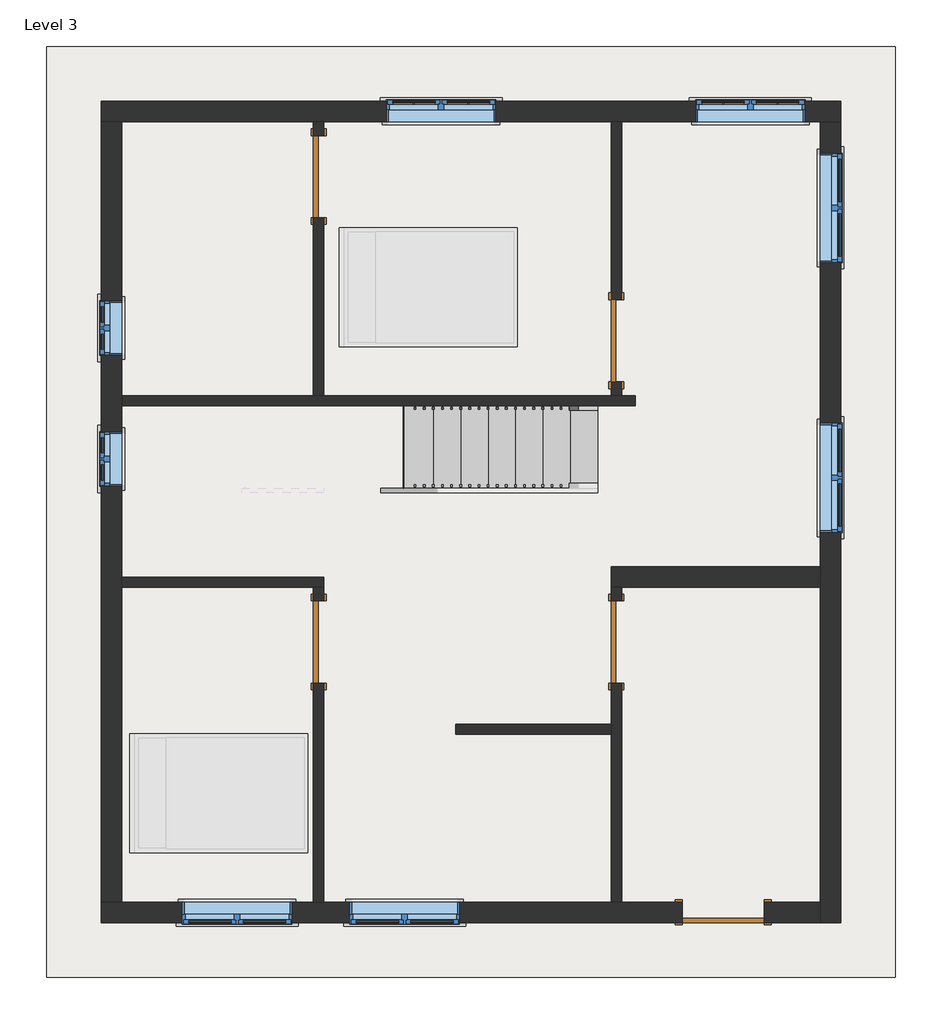
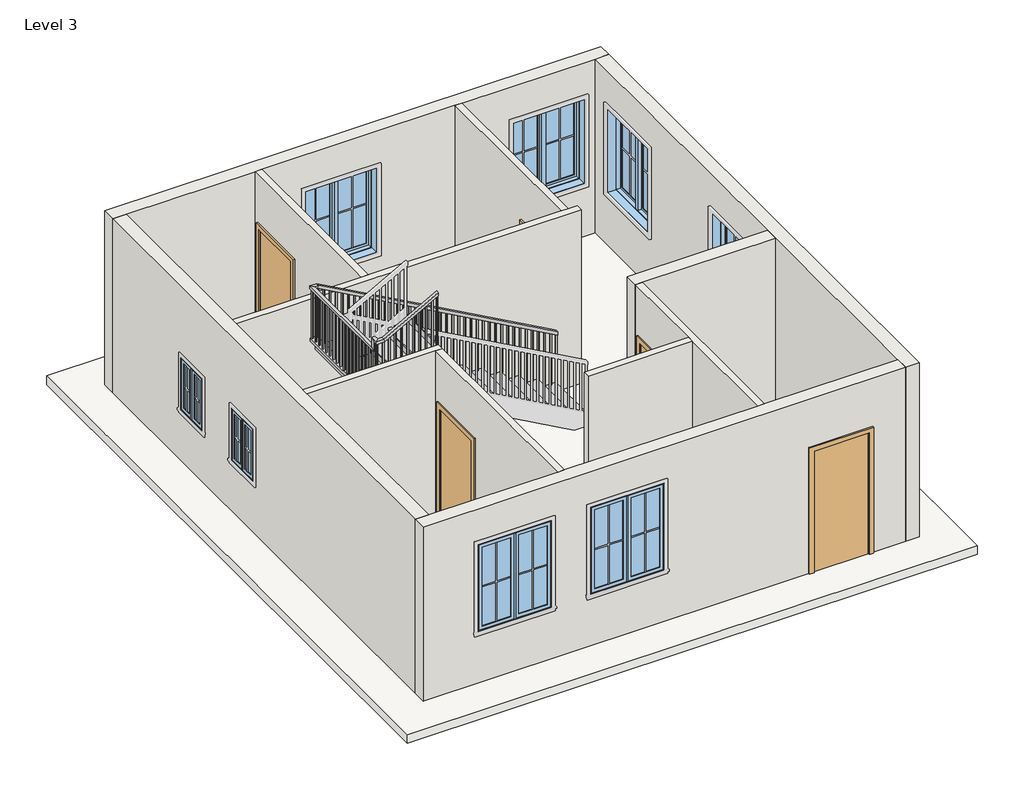
# One storey, part 1 of 2: 12 walls, 8 windows, 5 doors, 1 railing, 1 slab, 1 stair flight.
"""IFC4 building model written with IfcOpenShell, lengths in millimetres."""

from ifc_helpers import new_model, si_unit, frame, origin, place, context, project, spatial, polyline, outline, extrude, faceted_brep, transform, mapped, element, save
from components import door_e5f9f3c4, door_305aa2a5, door_0ca8825f, stair_flight_af090c4c, window_c417fced, window_8377141f

model = new_model("IFC4")

# Units and contexts
model_context = context("Model", 3, world=origin())
ifc_project = project(units=[si_unit("LENGTHUNIT", "METRE", prefix="MILLI")], contexts=[model_context])

# Site, building, storey
site = spatial("IfcSite", under=ifc_project)
building = spatial("IfcBuilding", under=site)
storey = spatial("IfcBuildingStorey", under=building, Name="Level 3", Elevation=6096.0)

# Doors
placement = place(None, origin())
door_shape = door_e5f9f3c4(model_context)
element("IfcDoor", 1, ObjectType="Single-Flush : 36\" x 84\"", at=placement, inside=storey, context=model_context, shape_type="MappedRepresentation", body=[
    mapped(door_shape, transform((3689.35, 13938.7372886, 6096.0), x_axis=(0.0, 1.0, 0.0), y_axis=(-1.0, 0.0, 0.0), z_axis=(0.0, 0.0, 1.0))),
])
door_2_shape = door_305aa2a5(model_context)
element("IfcDoor", 2, ObjectType="Single-Flush : 36\" x 84\"", at=placement, inside=storey, context=model_context, shape_type="MappedRepresentation", body=[
    mapped(door_2_shape, transform((7004.05, 12109.9372886, 6096.0), x_axis=(0.0, -1.0, 0.0), y_axis=(1.0, 0.0, 0.0), z_axis=(0.0, 0.0, 1.0))),
])
element("IfcDoor", 3, ObjectType="Single-Flush : 36\" x 84\"", at=placement, inside=storey, context=model_context, shape_type="MappedRepresentation", body=[
    mapped(door_2_shape, transform((3689.3519847, 8757.1372886, 6096.0), x_axis=(0.0, -1.0, 0.0), y_axis=(1.0, 0.0, 0.0), z_axis=(0.0, 0.0, 1.0))),
])
element("IfcDoor", 4, ObjectType="Single-Flush : 36\" x 84\"", at=placement, inside=storey, context=model_context, shape_type="MappedRepresentation", body=[
    mapped(door_2_shape, transform((7004.05, 8757.1372886, 6096.0), x_axis=(0.0, -1.0, 0.0), y_axis=(1.0, 0.0, 0.0), z_axis=(0.0, 0.0, 1.0))),
])
door_3_shape = door_0ca8825f(model_context)
element("IfcDoor", 5, ObjectType="Single-Flush : 36\" x 84\"", at=placement, inside=storey, context=model_context, shape_type="MappedRepresentation", body=[
    mapped(door_3_shape, transform((8194.675, 5747.2372886, 6096.0), x_axis=(-1.0, 0.0, 0.0), y_axis=(0.0, -1.0, 0.0), z_axis=(0.0, 0.0, 1.0))),
])

# Railing
element("IfcRailing", 6, ObjectType="Handrail - Rectangular", at=placement, inside=storey, context=model_context, shape_type="SolidModel", body=[
    faceted_brep([(6794.5, 11335.2372886, 7179.7333333), (6794.5, 11335.2372886, 7121.620221), (6794.5, 11386.0372886, 7121.620221), (6794.5, 11386.0372886, 7179.7333333), (2832.1, 11335.2372886, 9381.0666667), (2818.9363978, 11335.2372886, 9330.2666667), (2818.9363978, 11386.0372886, 9330.2666667), (2832.1, 11386.0372886, 9381.0666667), (2768.6, 11335.2372886, 9381.0666667), (2768.6, 11335.2372886, 9330.2666667), (2717.8, 11386.0372886, 9330.2666667), (2717.8, 11386.0372886, 9381.0666667), (2768.6, 9608.0372886, 9381.0666667), (2768.6, 9557.2372886, 9330.2666667), (2717.8, 9557.2372886, 9330.2666667), (2717.8, 9608.0372886, 9381.0666667), (2768.6, 9608.0372886, 9557.4555402), (2768.6, 9557.2372886, 9506.6555402), (2717.8, 9557.2372886, 9506.6555402), (2717.8, 9608.0372886, 9557.4555402), (2768.6, 9531.8372886, 9557.4555402), (2768.6, 9531.8372886, 9506.6555402), (2717.8, 9481.0372886, 9506.6555402), (2717.8, 9481.0372886, 9557.4555402), (2844.8, 9531.8372886, 9557.4555402), (2857.9635773, 9531.8372886, 9506.6555402), (2857.9635773, 9481.0372886, 9506.6555402), (2844.8, 9481.0372886, 9557.4555402), (3746.5019847, 9531.8372886, 10058.4), (3746.5019847, 9481.0372886, 10058.4), (3746.5019847, 9481.0372886, 10000.2869174), (3746.5019847, 9531.8372886, 10000.2869174)], [[[0, 1, 2, 3]], [[1, 0, 4, 5]], [[2, 1, 5, 6]], [[3, 2, 6, 7]], [[0, 3, 7, 4]], [[5, 4, 8, 9]], [[6, 5, 9, 10]], [[7, 6, 10, 11]], [[4, 7, 11, 8]], [[9, 8, 12, 13]], [[10, 9, 13, 14]], [[11, 10, 14, 15]], [[8, 11, 15, 12]], [[13, 12, 16, 17]], [[14, 13, 17, 18]], [[15, 14, 18, 19]], [[12, 15, 19, 16]], [[17, 16, 20, 21]], [[18, 17, 21, 22]], [[19, 18, 22, 23]], [[16, 19, 23, 20]], [[21, 20, 24, 25]], [[22, 21, 25, 26]], [[23, 22, 26, 27]], [[20, 23, 27, 24]], [[28, 29, 30, 31]], [[25, 24, 28, 31]], [[26, 25, 31, 30]], [[27, 26, 30, 29]], [[24, 27, 29, 28]]]),
    extrude(outline(polyline([(9956.1894234, 3667.125), (9945.606113, 3648.075), (8974.6666667, 3648.075), (8974.6666667, 3667.125), (9956.1894234, 3667.125)])), frame((0.0, 9496.9122886, 0.0), z_axis=(0.0, 1.0, 0.0), x_axis=(0.0, 0.0, 1.0)), (0.0, 0.0, 1.0), 19.05),
    extrude(outline(polyline([(9899.7451014, 3565.525), (9889.1617911, 3546.475), (8974.6666667, 3546.475), (8974.6666667, 3565.525), (9899.7451014, 3565.525)])), frame((0.0, 9496.9122886, 0.0), z_axis=(0.0, 1.0, 0.0), x_axis=(0.0, 0.0, 1.0)), (0.0, 0.0, 1.0), 19.05),
    extrude(outline(polyline([(9843.3007795, 3463.925), (9832.7174691, 3444.875), (8974.6666667, 3444.875), (8974.6666667, 3463.925), (9843.3007795, 3463.925)])), frame((0.0, 9496.9122886, 0.0), z_axis=(0.0, 1.0, 0.0), x_axis=(0.0, 0.0, 1.0)), (0.0, 0.0, 1.0), 19.05),
    extrude(outline(polyline([(9786.85609, 3362.325), (9776.2727797, 3343.275), (8805.3333333, 3343.275), (8805.3333333, 3362.325), (9786.85609, 3362.325)])), frame((0.0, 9496.9122886, 0.0), z_axis=(0.0, 1.0, 0.0), x_axis=(0.0, 0.0, 1.0)), (0.0, 0.0, 1.0), 19.05),
    extrude(outline(polyline([(9730.4117681, 3260.725), (9719.8284577, 3241.675), (8805.3333333, 3241.675), (8805.3333333, 3260.725), (9730.4117681, 3260.725)])), frame((0.0, 9496.9122886, 0.0), z_axis=(0.0, 1.0, 0.0), x_axis=(0.0, 0.0, 1.0)), (0.0, 0.0, 1.0), 19.05),
    extrude(outline(polyline([(9673.9674462, 3159.125), (9663.3841358, 3140.075), (8805.3333333, 3140.075), (8805.3333333, 3159.125), (9673.9674462, 3159.125)])), frame((0.0, 9496.9122886, 0.0), z_axis=(0.0, 1.0, 0.0), x_axis=(0.0, 0.0, 1.0)), (0.0, 0.0, 1.0), 19.05),
    extrude(outline(polyline([(9617.5227567, 3057.525), (9606.9394463, 3038.475), (8636.0, 3038.475), (8636.0, 3057.525), (9617.5227567, 3057.525)])), frame((0.0, 9496.9122886, 0.0), z_axis=(0.0, 1.0, 0.0), x_axis=(0.0, 0.0, 1.0)), (0.0, 0.0, 1.0), 19.05),
    extrude(outline(polyline([(9561.0784348, 2955.925), (9550.4951244, 2936.875), (8636.0, 2936.875), (8636.0, 2955.925), (9561.0784348, 2955.925)])), frame((0.0, 9496.9122886, 0.0), z_axis=(0.0, 1.0, 0.0), x_axis=(0.0, 0.0, 1.0)), (0.0, 0.0, 1.0), 19.05),
    extrude(outline(polyline([(9504.6341128, 2854.325), (9494.0508025, 2835.275), (8636.0, 2835.275), (8636.0, 2854.325), (9504.6341128, 2854.325)])), frame((0.0, 9496.9122886, 0.0), z_axis=(0.0, 1.0, 0.0), x_axis=(0.0, 0.0, 1.0)), (0.0, 0.0, 1.0), 19.05),
    extrude(outline(polyline([(2733.675, 9541.3622886), (2752.725, 9541.3622886), (2752.725, 9522.3122886), (2733.675, 9522.3122886), (2733.675, 9541.3622886)])), frame((0.0, 0.0, 8466.6666667), z_axis=(0.0, 0.0, 1.0), x_axis=(1.0, 0.0, 0.0)), (0.0, 0.0, 1.0), 1039.9888736),
    extrude(outline(polyline([(2733.675, 9642.9622886), (2752.725, 9642.9622886), (2752.725, 9623.9122886), (2733.675, 9623.9122886), (2733.675, 9642.9622886)])), frame((0.0, 0.0, 8466.6666667), z_axis=(0.0, 0.0, 1.0), x_axis=(1.0, 0.0, 0.0)), (0.0, 0.0, 1.0), 863.6),
    extrude(outline(polyline([(2733.675, 9744.5622886), (2752.725, 9744.5622886), (2752.725, 9725.5122886), (2733.675, 9725.5122886), (2733.675, 9744.5622886)])), frame((0.0, 0.0, 8466.6666667), z_axis=(0.0, 0.0, 1.0), x_axis=(1.0, 0.0, 0.0)), (0.0, 0.0, 1.0), 863.6),
    extrude(outline(polyline([(2733.675, 9846.1622886), (2752.725, 9846.1622886), (2752.725, 9827.1122886), (2733.675, 9827.1122886), (2733.675, 9846.1622886)])), frame((0.0, 0.0, 8466.6666667), z_axis=(0.0, 0.0, 1.0), x_axis=(1.0, 0.0, 0.0)), (0.0, 0.0, 1.0), 863.6),
    extrude(outline(polyline([(2733.675, 9947.7622886), (2752.725, 9947.7622886), (2752.725, 9928.7122886), (2733.675, 9928.7122886), (2733.675, 9947.7622886)])), frame((0.0, 0.0, 8466.6666667), z_axis=(0.0, 0.0, 1.0), x_axis=(1.0, 0.0, 0.0)), (0.0, 0.0, 1.0), 863.6),
    extrude(outline(polyline([(2733.675, 10049.3622886), (2752.725, 10049.3622886), (2752.725, 10030.3122886), (2733.675, 10030.3122886), (2733.675, 10049.3622886)])), frame((0.0, 0.0, 8466.6666667), z_axis=(0.0, 0.0, 1.0), x_axis=(1.0, 0.0, 0.0)), (0.0, 0.0, 1.0), 863.6),
    extrude(outline(polyline([(2733.675, 10150.9622886), (2752.725, 10150.9622886), (2752.725, 10131.9122886), (2733.675, 10131.9122886), (2733.675, 10150.9622886)])), frame((0.0, 0.0, 8466.6666667), z_axis=(0.0, 0.0, 1.0), x_axis=(1.0, 0.0, 0.0)), (0.0, 0.0, 1.0), 863.6),
    extrude(outline(polyline([(2733.675, 10252.5622886), (2752.725, 10252.5622886), (2752.725, 10233.5122886), (2733.675, 10233.5122886), (2733.675, 10252.5622886)])), frame((0.0, 0.0, 8466.6666667), z_axis=(0.0, 0.0, 1.0), x_axis=(1.0, 0.0, 0.0)), (0.0, 0.0, 1.0), 863.6),
    extrude(outline(polyline([(2733.675, 10354.1622886), (2752.725, 10354.1622886), (2752.725, 10335.1122886), (2733.675, 10335.1122886), (2733.675, 10354.1622886)])), frame((0.0, 0.0, 8466.6666667), z_axis=(0.0, 0.0, 1.0), x_axis=(1.0, 0.0, 0.0)), (0.0, 0.0, 1.0), 863.6),
    extrude(outline(polyline([(2733.675, 10455.7622886), (2752.725, 10455.7622886), (2752.725, 10436.7122886), (2733.675, 10436.7122886), (2733.675, 10455.7622886)])), frame((0.0, 0.0, 8466.6666667), z_axis=(0.0, 0.0, 1.0), x_axis=(1.0, 0.0, 0.0)), (0.0, 0.0, 1.0), 863.6),
    extrude(outline(polyline([(2733.675, 10557.3622886), (2752.725, 10557.3622886), (2752.725, 10538.3122886), (2733.675, 10538.3122886), (2733.675, 10557.3622886)])), frame((0.0, 0.0, 8466.6666667), z_axis=(0.0, 0.0, 1.0), x_axis=(1.0, 0.0, 0.0)), (0.0, 0.0, 1.0), 863.6),
    extrude(outline(polyline([(2733.675, 10658.9622886), (2752.725, 10658.9622886), (2752.725, 10639.9122886), (2733.675, 10639.9122886), (2733.675, 10658.9622886)])), frame((0.0, 0.0, 8466.6666667), z_axis=(0.0, 0.0, 1.0), x_axis=(1.0, 0.0, 0.0)), (0.0, 0.0, 1.0), 863.6),
    extrude(outline(polyline([(2733.675, 10760.5622886), (2752.725, 10760.5622886), (2752.725, 10741.5122886), (2733.675, 10741.5122886), (2733.675, 10760.5622886)])), frame((0.0, 0.0, 8466.6666667), z_axis=(0.0, 0.0, 1.0), x_axis=(1.0, 0.0, 0.0)), (0.0, 0.0, 1.0), 863.6),
    extrude(outline(polyline([(2733.675, 10862.1622886), (2752.725, 10862.1622886), (2752.725, 10843.1122886), (2733.675, 10843.1122886), (2733.675, 10862.1622886)])), frame((0.0, 0.0, 8466.6666667), z_axis=(0.0, 0.0, 1.0), x_axis=(1.0, 0.0, 0.0)), (0.0, 0.0, 1.0), 863.6),
    extrude(outline(polyline([(2733.675, 10963.7622886), (2752.725, 10963.7622886), (2752.725, 10944.7122886), (2733.675, 10944.7122886), (2733.675, 10963.7622886)])), frame((0.0, 0.0, 8466.6666667), z_axis=(0.0, 0.0, 1.0), x_axis=(1.0, 0.0, 0.0)), (0.0, 0.0, 1.0), 863.6),
    extrude(outline(polyline([(2733.675, 11065.3622886), (2752.725, 11065.3622886), (2752.725, 11046.3122886), (2733.675, 11046.3122886), (2733.675, 11065.3622886)])), frame((0.0, 0.0, 8466.6666667), z_axis=(0.0, 0.0, 1.0), x_axis=(1.0, 0.0, 0.0)), (0.0, 0.0, 1.0), 863.6),
    extrude(outline(polyline([(2733.675, 11166.9622886), (2752.725, 11166.9622886), (2752.725, 11147.9122886), (2733.675, 11147.9122886), (2733.675, 11166.9622886)])), frame((0.0, 0.0, 8466.6666667), z_axis=(0.0, 0.0, 1.0), x_axis=(1.0, 0.0, 0.0)), (0.0, 0.0, 1.0), 863.6),
    extrude(outline(polyline([(2733.675, 11268.5622886), (2752.725, 11268.5622886), (2752.725, 11249.5122886), (2733.675, 11249.5122886), (2733.675, 11268.5622886)])), frame((0.0, 0.0, 8466.6666667), z_axis=(0.0, 0.0, 1.0), x_axis=(1.0, 0.0, 0.0)), (0.0, 0.0, 1.0), 863.6),
    extrude(outline(polyline([(9317.6618876, 2841.625), (9328.245221, 2822.575), (8466.6666667, 2822.575), (8466.6666667, 2841.625), (9317.6618876, 2841.625)])), frame((0.0, 11351.1122886, 0.0), z_axis=(0.0, 1.0, 0.0), x_axis=(0.0, 0.0, 1.0)), (0.0, 0.0, 1.0), 19.05),
    extrude(outline(polyline([(9261.2174432, 2943.225), (9271.8007765, 2924.175), (8297.3333333, 2924.175), (8297.3333333, 2943.225), (9261.2174432, 2943.225)])), frame((0.0, 11351.1122886, 0.0), z_axis=(0.0, 1.0, 0.0), x_axis=(0.0, 0.0, 1.0)), (0.0, 0.0, 1.0), 19.05),
    extrude(outline(polyline([(9204.7729988, 3044.825), (9215.3563321, 3025.775), (8297.3333333, 3025.775), (8297.3333333, 3044.825), (9204.7729988, 3044.825)])), frame((0.0, 11351.1122886, 0.0), z_axis=(0.0, 1.0, 0.0), x_axis=(0.0, 0.0, 1.0)), (0.0, 0.0, 1.0), 19.05),
    extrude(outline(polyline([(9148.3285543, 3146.425), (9158.9118876, 3127.375), (8297.3333333, 3127.375), (8297.3333333, 3146.425), (9148.3285543, 3146.425)])), frame((0.0, 11351.1122886, 0.0), z_axis=(0.0, 1.0, 0.0), x_axis=(0.0, 0.0, 1.0)), (0.0, 0.0, 1.0), 19.05),
    extrude(outline(polyline([(9091.8841099, 3248.025), (9102.4674432, 3228.975), (8128.0, 3228.975), (8128.0, 3248.025), (9091.8841099, 3248.025)])), frame((0.0, 11351.1122886, 0.0), z_axis=(0.0, 1.0, 0.0), x_axis=(0.0, 0.0, 1.0)), (0.0, 0.0, 1.0), 19.05),
    extrude(outline(polyline([(9035.4396654, 3349.625), (9046.0229988, 3330.575), (8128.0, 3330.575), (8128.0, 3349.625), (9035.4396654, 3349.625)])), frame((0.0, 11351.1122886, 0.0), z_axis=(0.0, 1.0, 0.0), x_axis=(0.0, 0.0, 1.0)), (0.0, 0.0, 1.0), 19.05),
    extrude(outline(polyline([(8978.995221, 3451.225), (8989.5785543, 3432.175), (8128.0, 3432.175), (8128.0, 3451.225), (8978.995221, 3451.225)])), frame((0.0, 11351.1122886, 0.0), z_axis=(0.0, 1.0, 0.0), x_axis=(0.0, 0.0, 1.0)), (0.0, 0.0, 1.0), 19.05),
    extrude(outline(polyline([(8922.5507765, 3552.825), (8933.1341099, 3533.775), (7958.6666667, 3533.775), (7958.6666667, 3552.825), (8922.5507765, 3552.825)])), frame((0.0, 11351.1122886, 0.0), z_axis=(0.0, 1.0, 0.0), x_axis=(0.0, 0.0, 1.0)), (0.0, 0.0, 1.0), 19.05),
    extrude(outline(polyline([(8866.1063321, 3654.425), (8876.6896654, 3635.375), (7958.6666667, 3635.375), (7958.6666667, 3654.425), (8866.1063321, 3654.425)])), frame((0.0, 11351.1122886, 0.0), z_axis=(0.0, 1.0, 0.0), x_axis=(0.0, 0.0, 1.0)), (0.0, 0.0, 1.0), 19.05),
    extrude(outline(polyline([(8809.6618876, 3756.025), (8820.245221, 3736.975), (7958.6666667, 3736.975), (7958.6666667, 3756.025), (8809.6618876, 3756.025)])), frame((0.0, 11351.1122886, 0.0), z_axis=(0.0, 1.0, 0.0), x_axis=(0.0, 0.0, 1.0)), (0.0, 0.0, 1.0), 19.05),
    extrude(outline(polyline([(8753.2174432, 3857.625), (8763.8007765, 3838.575), (7789.3333333, 3838.575), (7789.3333333, 3857.625), (8753.2174432, 3857.625)])), frame((0.0, 11351.1122886, 0.0), z_axis=(0.0, 1.0, 0.0), x_axis=(0.0, 0.0, 1.0)), (0.0, 0.0, 1.0), 19.05),
    extrude(outline(polyline([(8696.7729988, 3959.225), (8707.3563321, 3940.175), (7789.3333333, 3940.175), (7789.3333333, 3959.225), (8696.7729988, 3959.225)])), frame((0.0, 11351.1122886, 0.0), z_axis=(0.0, 1.0, 0.0), x_axis=(0.0, 0.0, 1.0)), (0.0, 0.0, 1.0), 19.05),
    extrude(outline(polyline([(8640.3285543, 4060.825), (8650.9118876, 4041.775), (7789.3333333, 4041.775), (7789.3333333, 4060.825), (8640.3285543, 4060.825)])), frame((0.0, 11351.1122886, 0.0), z_axis=(0.0, 1.0, 0.0), x_axis=(0.0, 0.0, 1.0)), (0.0, 0.0, 1.0), 19.05),
    extrude(outline(polyline([(8583.8841099, 4162.425), (8594.4674432, 4143.375), (7620.0, 4143.375), (7620.0, 4162.425), (8583.8841099, 4162.425)])), frame((0.0, 11351.1122886, 0.0), z_axis=(0.0, 1.0, 0.0), x_axis=(0.0, 0.0, 1.0)), (0.0, 0.0, 1.0), 19.05),
    extrude(outline(polyline([(8527.4396654, 4264.025), (8538.0229988, 4244.975), (7620.0, 4244.975), (7620.0, 4264.025), (8527.4396654, 4264.025)])), frame((0.0, 11351.1122886, 0.0), z_axis=(0.0, 1.0, 0.0), x_axis=(0.0, 0.0, 1.0)), (0.0, 0.0, 1.0), 19.05),
    extrude(outline(polyline([(8470.995221, 4365.625), (8481.5785543, 4346.575), (7620.0, 4346.575), (7620.0, 4365.625), (8470.995221, 4365.625)])), frame((0.0, 11351.1122886, 0.0), z_axis=(0.0, 1.0, 0.0), x_axis=(0.0, 0.0, 1.0)), (0.0, 0.0, 1.0), 19.05),
    extrude(outline(polyline([(8414.5507765, 4467.225), (8425.1341099, 4448.175), (7450.6666667, 4448.175), (7450.6666667, 4467.225), (8414.5507765, 4467.225)])), frame((0.0, 11351.1122886, 0.0), z_axis=(0.0, 1.0, 0.0), x_axis=(0.0, 0.0, 1.0)), (0.0, 0.0, 1.0), 19.05),
    extrude(outline(polyline([(8358.1063321, 4568.825), (8368.6896654, 4549.775), (7450.6666667, 4549.775), (7450.6666667, 4568.825), (8358.1063321, 4568.825)])), frame((0.0, 11351.1122886, 0.0), z_axis=(0.0, 1.0, 0.0), x_axis=(0.0, 0.0, 1.0)), (0.0, 0.0, 1.0), 19.05),
    extrude(outline(polyline([(8301.6618876, 4670.425), (8312.245221, 4651.375), (7450.6666667, 4651.375), (7450.6666667, 4670.425), (8301.6618876, 4670.425)])), frame((0.0, 11351.1122886, 0.0), z_axis=(0.0, 1.0, 0.0), x_axis=(0.0, 0.0, 1.0)), (0.0, 0.0, 1.0), 19.05),
    extrude(outline(polyline([(8245.2174432, 4772.025), (8255.8007765, 4752.975), (7281.3333333, 4752.975), (7281.3333333, 4772.025), (8245.2174432, 4772.025)])), frame((0.0, 11351.1122886, 0.0), z_axis=(0.0, 1.0, 0.0), x_axis=(0.0, 0.0, 1.0)), (0.0, 0.0, 1.0), 19.05),
    extrude(outline(polyline([(8188.7729988, 4873.625), (8199.3563321, 4854.575), (7281.3333333, 4854.575), (7281.3333333, 4873.625), (8188.7729988, 4873.625)])), frame((0.0, 11351.1122886, 0.0), z_axis=(0.0, 1.0, 0.0), x_axis=(0.0, 0.0, 1.0)), (0.0, 0.0, 1.0), 19.05),
    extrude(outline(polyline([(8132.3285543, 4975.225), (8142.9118876, 4956.175), (7281.3333333, 4956.175), (7281.3333333, 4975.225), (8132.3285543, 4975.225)])), frame((0.0, 11351.1122886, 0.0), z_axis=(0.0, 1.0, 0.0), x_axis=(0.0, 0.0, 1.0)), (0.0, 0.0, 1.0), 19.05),
    extrude(outline(polyline([(8075.8841099, 5076.825), (8086.4674432, 5057.775), (7112.0, 5057.775), (7112.0, 5076.825), (8075.8841099, 5076.825)])), frame((0.0, 11351.1122886, 0.0), z_axis=(0.0, 1.0, 0.0), x_axis=(0.0, 0.0, 1.0)), (0.0, 0.0, 1.0), 19.05),
    extrude(outline(polyline([(8019.4396654, 5178.425), (8030.0229988, 5159.375), (7112.0, 5159.375), (7112.0, 5178.425), (8019.4396654, 5178.425)])), frame((0.0, 11351.1122886, 0.0), z_axis=(0.0, 1.0, 0.0), x_axis=(0.0, 0.0, 1.0)), (0.0, 0.0, 1.0), 19.05),
    extrude(outline(polyline([(7962.995221, 5280.025), (7973.5785543, 5260.975), (7112.0, 5260.975), (7112.0, 5280.025), (7962.995221, 5280.025)])), frame((0.0, 11351.1122886, 0.0), z_axis=(0.0, 1.0, 0.0), x_axis=(0.0, 0.0, 1.0)), (0.0, 0.0, 1.0), 19.05),
    extrude(outline(polyline([(7906.5507765, 5381.625), (7917.1341099, 5362.575), (6942.6666667, 5362.575), (6942.6666667, 5381.625), (7906.5507765, 5381.625)])), frame((0.0, 11351.1122886, 0.0), z_axis=(0.0, 1.0, 0.0), x_axis=(0.0, 0.0, 1.0)), (0.0, 0.0, 1.0), 19.05),
    extrude(outline(polyline([(7850.1063321, 5483.225), (7860.6896654, 5464.175), (6942.6666667, 5464.175), (6942.6666667, 5483.225), (7850.1063321, 5483.225)])), frame((0.0, 11351.1122886, 0.0), z_axis=(0.0, 1.0, 0.0), x_axis=(0.0, 0.0, 1.0)), (0.0, 0.0, 1.0), 19.05),
    extrude(outline(polyline([(7793.6618876, 5584.825), (7804.245221, 5565.775), (6942.6666667, 5565.775), (6942.6666667, 5584.825), (7793.6618876, 5584.825)])), frame((0.0, 11351.1122886, 0.0), z_axis=(0.0, 1.0, 0.0), x_axis=(0.0, 0.0, 1.0)), (0.0, 0.0, 1.0), 19.05),
    extrude(outline(polyline([(7737.2174432, 5686.425), (7747.8007765, 5667.375), (6773.3333333, 5667.375), (6773.3333333, 5686.425), (7737.2174432, 5686.425)])), frame((0.0, 11351.1122886, 0.0), z_axis=(0.0, 1.0, 0.0), x_axis=(0.0, 0.0, 1.0)), (0.0, 0.0, 1.0), 19.05),
    extrude(outline(polyline([(7680.7729988, 5788.025), (7691.3563321, 5768.975), (6773.3333333, 5768.975), (6773.3333333, 5788.025), (7680.7729988, 5788.025)])), frame((0.0, 11351.1122886, 0.0), z_axis=(0.0, 1.0, 0.0), x_axis=(0.0, 0.0, 1.0)), (0.0, 0.0, 1.0), 19.05),
    extrude(outline(polyline([(7624.3285543, 5889.625), (7634.9118876, 5870.575), (6773.3333333, 5870.575), (6773.3333333, 5889.625), (7624.3285543, 5889.625)])), frame((0.0, 11351.1122886, 0.0), z_axis=(0.0, 1.0, 0.0), x_axis=(0.0, 0.0, 1.0)), (0.0, 0.0, 1.0), 19.05),
    extrude(outline(polyline([(7567.8841099, 5991.225), (7578.4674432, 5972.175), (6604.0, 5972.175), (6604.0, 5991.225), (7567.8841099, 5991.225)])), frame((0.0, 11351.1122886, 0.0), z_axis=(0.0, 1.0, 0.0), x_axis=(0.0, 0.0, 1.0)), (0.0, 0.0, 1.0), 19.05),
    extrude(outline(polyline([(7511.4396654, 6092.825), (7522.0229988, 6073.775), (6604.0, 6073.775), (6604.0, 6092.825), (7511.4396654, 6092.825)])), frame((0.0, 11351.1122886, 0.0), z_axis=(0.0, 1.0, 0.0), x_axis=(0.0, 0.0, 1.0)), (0.0, 0.0, 1.0), 19.05),
    extrude(outline(polyline([(7454.995221, 6194.425), (7465.5785543, 6175.375), (6604.0, 6175.375), (6604.0, 6194.425), (7454.995221, 6194.425)])), frame((0.0, 11351.1122886, 0.0), z_axis=(0.0, 1.0, 0.0), x_axis=(0.0, 0.0, 1.0)), (0.0, 0.0, 1.0), 19.05),
    extrude(outline(polyline([(7398.5507765, 6296.025), (7409.1341099, 6276.975), (6434.6666667, 6276.975), (6434.6666667, 6296.025), (7398.5507765, 6296.025)])), frame((0.0, 11351.1122886, 0.0), z_axis=(0.0, 1.0, 0.0), x_axis=(0.0, 0.0, 1.0)), (0.0, 0.0, 1.0), 19.05),
    extrude(outline(polyline([(7342.1063321, 6397.625), (7352.6896654, 6378.575), (6434.6666667, 6378.575), (6434.6666667, 6397.625), (7342.1063321, 6397.625)])), frame((0.0, 11351.1122886, 0.0), z_axis=(0.0, 1.0, 0.0), x_axis=(0.0, 0.0, 1.0)), (0.0, 0.0, 1.0), 19.05),
    extrude(outline(polyline([(7285.6618876, 6499.225), (7296.245221, 6480.175), (6434.6666667, 6480.175), (6434.6666667, 6499.225), (7285.6618876, 6499.225)])), frame((0.0, 11351.1122886, 0.0), z_axis=(0.0, 1.0, 0.0), x_axis=(0.0, 0.0, 1.0)), (0.0, 0.0, 1.0), 19.05),
    extrude(outline(polyline([(7229.2174432, 6600.825), (7239.8007765, 6581.775), (6265.3333333, 6581.775), (6265.3333333, 6600.825), (7229.2174432, 6600.825)])), frame((0.0, 11351.1122886, 0.0), z_axis=(0.0, 1.0, 0.0), x_axis=(0.0, 0.0, 1.0)), (0.0, 0.0, 1.0), 19.05),
    extrude(outline(polyline([(7172.7729988, 6702.425), (7183.3563321, 6683.375), (6265.3333333, 6683.375), (6265.3333333, 6702.425), (7172.7729988, 6702.425)])), frame((0.0, 11351.1122886, 0.0), z_axis=(0.0, 1.0, 0.0), x_axis=(0.0, 0.0, 1.0)), (0.0, 0.0, 1.0), 19.05),
    extrude(outline(polyline([(2733.675, 9515.9622886), (2752.725, 9515.9622886), (2752.725, 9496.9122886), (2733.675, 9496.9122886), (2733.675, 9515.9622886)])), frame((0.0, 0.0, 8466.6666667), z_axis=(0.0, 0.0, 1.0), x_axis=(1.0, 0.0, 0.0)), (0.0, 0.0, 1.0), 1039.9888736),
    extrude(outline(polyline([(2752.725, 11370.1622886), (2752.725, 11351.1122886), (2733.675, 11351.1122886), (2733.675, 11370.1622886), (2752.725, 11370.1622886)])), frame((0.0, 0.0, 8466.6666667), z_axis=(0.0, 0.0, 1.0), x_axis=(1.0, 0.0, 0.0)), (0.0, 0.0, 1.0), 863.6),
    extrude(outline(polyline([(10000.2869174, 3746.5019847), (9989.703607, 3727.4519847), (8974.6666667, 3727.4519847), (8974.6666667, 3746.5019847), (10000.2869174, 3746.5019847)])), frame((0.0, 9496.9122886, 0.0), z_axis=(0.0, 1.0, 0.0), x_axis=(0.0, 0.0, 1.0)), (0.0, 0.0, 1.0), 19.05),
    extrude(outline(polyline([(7121.620221, 6794.5), (7132.2035543, 6775.45), (6265.3333333, 6775.45), (6265.3333333, 6794.5), (7121.620221, 6794.5)])), frame((0.0, 11351.1122886, 0.0), z_axis=(0.0, 1.0, 0.0), x_axis=(0.0, 0.0, 1.0)), (0.0, 0.0, 1.0), 19.05),
])

# Slab
element("IfcSlab", 7, ObjectType="Generic - 12\"", at=placement, inside=storey, context=model_context, shape_type="SweptSolid", body=[
    extrude(outline(polyline([(10109.2, 15386.5372886), (10109.2, 5023.3372886), (660.4, 5023.3372886), (660.4, 15386.5372886), (10109.2, 15386.5372886)])), frame((0.0, 0.0, 5943.6), z_axis=(0.0, 0.0, 1.0), x_axis=(1.0, 0.0, 0.0)), (0.0, 0.0, 1.0), 152.4),
])

# Stair flight
stair_flight_shape = stair_flight_af090c4c(model_context)
element("IfcStairFlight", 8, ObjectType="2\" Tread 1\" Nosing 1/4\" Riser", at=placement, inside=storey, context=model_context, shape_type="MappedRepresentation", body=[
    mapped(stair_flight_shape, transform((0.0, 0.0, 0.0), x_axis=(1.0, 0.0, 0.0), y_axis=(0.0, 1.0, 0.0), z_axis=(0.0, 0.0, 1.0))),
])

# Walls
element("IfcWall", 9, ObjectType="Generic - 5\"", at=placement, inside=storey, context=model_context, shape_type="SweptSolid", body=[
    extrude(outline(polyline([(14548.3372886, 6096.0), (14395.9372886, 6096.0), (14395.9372886, 8229.6), (13481.5372886, 8229.6), (13481.5372886, 6096.0), (11500.3372886, 6096.0), (11500.3372886, 9144.0), (14548.3372886, 9144.0), (14548.3372886, 6096.0)])), frame((3632.2, 0.0, 0.0), z_axis=(1.0, 0.0, 0.0), x_axis=(0.0, 1.0, 0.0)), (0.0, 0.0, 1.0), 114.3),
])
element("IfcWall", 10, ObjectType="Generic - 5\"", at=placement, inside=storey, context=model_context, shape_type="SweptSolid", body=[
    extrude(outline(polyline([(11652.7372886, 8229.6), (11652.7372886, 6096.0), (11500.3372886, 6096.0), (11500.3372886, 9144.0), (14548.3372886, 9144.0), (14548.3372886, 6096.0), (12567.1372886, 6096.0), (12567.1372886, 8229.6), (11652.7372886, 8229.6)])), frame((6946.9, 0.0, 0.0), z_axis=(1.0, 0.0, 0.0), x_axis=(0.0, 1.0, 0.0)), (0.0, 0.0, 1.0), 114.3),
])
element("IfcWall", 11, ObjectType="Generic - 5\"", at=placement, inside=storey, context=model_context, shape_type="Brep", body=[
    faceted_brep([(1498.6, 11386.0372886, 6096.0), (7213.6, 11386.0372886, 6096.0), (7213.6, 11386.0372886, 9144.0), (1498.6, 11386.0372886, 9144.0), (1498.6, 11500.3372886, 6096.0), (1498.6, 11500.3372886, 9144.0), (3632.2, 11500.3372886, 9144.0), (3746.5, 11500.3372886, 9144.0), (6946.9, 11500.3372886, 9144.0), (7061.2, 11500.3372886, 9144.0), (7213.6, 11500.3372886, 9144.0), (7213.6, 11500.3372886, 6096.0), (7061.2, 11500.3372886, 6096.0), (6946.9, 11500.3372886, 6096.0), (3746.5, 11500.3372886, 6096.0), (3632.2, 11500.3372886, 6096.0)], [[[0, 1, 2, 3]], [[4, 5, 6, 7, 8, 9, 10, 11, 12, 13, 14, 15]], [[1, 0, 4, 15, 14, 13, 12, 11]], [[2, 1, 11, 10]], [[3, 2, 10, 9, 8, 7, 6, 5]], [[0, 3, 5, 4]]]),
])
element("IfcWall", 12, ObjectType="Generic - 5\"", at=placement, inside=storey, context=model_context, shape_type="Brep", body=[
    faceted_brep([(1498.6, 9366.7372886, 6096.0), (3632.2019847, 9366.7372886, 6096.0), (3746.5019847, 9366.7372886, 6096.0), (3746.5019847, 9366.7372886, 9144.0), (3632.2019847, 9366.7372886, 9144.0), (1498.6, 9366.7372886, 9144.0), (1498.6, 9481.0372886, 6096.0), (1498.6, 9481.0372886, 9144.0), (3746.5019847, 9481.0372886, 9144.0), (3746.5019847, 9481.0372886, 6096.0)], [[[0, 1, 2, 3, 4, 5]], [[6, 7, 8, 9]], [[2, 1, 0, 6, 9]], [[5, 4, 3, 8, 7]], [[0, 5, 7, 6]], [[3, 2, 9, 8]]]),
])
element("IfcWall", 13, ObjectType="Generic - 5\"", at=placement, inside=storey, context=model_context, shape_type="SweptSolid", body=[
    extrude(outline(polyline([(8299.9372886, 8229.6), (8299.9372886, 6096.0), (5861.5372886, 6096.0), (5861.5372886, 9144.0), (9366.7372886, 9144.0), (9366.7372886, 6096.0), (9214.3372886, 6096.0), (9214.3372886, 8229.6), (8299.9372886, 8229.6)])), frame((3632.2019847, 0.0, 0.0), z_axis=(1.0, 0.0, 0.0), x_axis=(0.0, 1.0, 0.0)), (0.0, 0.0, 1.0), 114.3),
])
element("IfcWall", 14, ObjectType="Generic - 5\"", at=placement, inside=storey, context=model_context, shape_type="Brep", body=[
    faceted_brep([(7061.2, 5861.5372886, 6096.0), (7061.2, 8299.9372886, 6096.0), (7061.2, 8299.9372886, 8229.6), (7061.2, 9214.3372886, 8229.6), (7061.2, 9214.3372886, 6096.0), (7061.2, 9366.7372886, 6096.0), (7061.2, 9366.7372886, 9144.0), (7061.2, 5861.5372886, 9144.0), (6946.9, 8299.9372886, 8229.6), (6946.9, 8299.9372886, 6096.0), (6946.9, 7842.7372886, 6096.0), (6946.9, 7728.4372886, 6096.0), (6946.9, 5861.5372886, 6096.0), (6946.9, 5861.5372886, 9144.0), (6946.9, 7728.4372886, 9144.0), (6946.9, 7842.7372886, 9144.0), (6946.9, 9366.7372886, 9144.0), (6946.9, 9366.7372886, 6096.0), (6946.9, 9214.3372886, 6096.0), (6946.9, 9214.3372886, 8229.6)], [[[0, 1, 2, 3, 4, 5, 6, 7]], [[8, 9, 10, 11, 12, 13, 14, 15, 16, 17, 18, 19]], [[18, 17, 5, 4]], [[12, 11, 10, 9, 1, 0]], [[7, 6, 16, 15, 14, 13]], [[0, 7, 13, 12]], [[6, 5, 17, 16]], [[2, 1, 9, 8]], [[3, 2, 8, 19]], [[4, 3, 19, 18]]]),
])
element("IfcWall", 15, ObjectType="Generic - 5\"", at=placement, inside=storey, context=model_context, shape_type="SweptSolid", body=[
    extrude(outline(polyline([(5215.2207778, 7842.7372886), (6946.9, 7842.7372886), (6946.9, 7728.4372886), (5215.2207778, 7728.4372886), (5215.2207778, 7842.7372886)])), frame((0.0, 0.0, 6096.0), z_axis=(0.0, 0.0, 1.0), x_axis=(1.0, 0.0, 0.0)), (0.0, 0.0, 1.0), 3048.0),
])
element("IfcWall", 16, ObjectType="Generic - 8\"", at=placement, inside=storey, context=model_context, shape_type="Brep", body=[
    faceted_brep([(1270.0, 14548.3372886, 6096.0), (1498.6, 14548.3372886, 6096.0), (3632.2, 14548.3372886, 6096.0), (3746.5, 14548.3372886, 6096.0), (6946.9, 14548.3372886, 6096.0), (7061.2, 14548.3372886, 6096.0), (9271.0, 14548.3372886, 6096.0), (9499.6, 14548.3372886, 6096.0), (9499.6, 14548.3372886, 9144.0), (9271.0, 14548.3372886, 9144.0), (7061.2, 14548.3372886, 9144.0), (6946.9, 14548.3372886, 9144.0), (3746.5, 14548.3372886, 9144.0), (3632.2, 14548.3372886, 9144.0), (1498.6, 14548.3372886, 9144.0), (1270.0, 14548.3372886, 9144.0), (9105.9, 14548.3372886, 8534.4), (9105.9, 14548.3372886, 7010.4), (7886.7, 14548.3372886, 7010.4), (7886.7, 14548.3372886, 8534.4), (5662.6125, 14548.3372886, 8534.4), (5662.6125, 14548.3372886, 7010.4), (4443.4125, 14548.3372886, 7010.4), (4443.4125, 14548.3372886, 8534.4), (1270.0, 14776.9372886, 6096.0), (1270.0, 14776.9372886, 9144.0), (9499.6, 14776.9372886, 9144.0), (9499.6, 14776.9372886, 6096.0), (9105.9, 14776.9372886, 8534.4), (7886.7, 14776.9372886, 8534.4), (7886.7, 14776.9372886, 7010.4), (9105.9, 14776.9372886, 7010.4), (5662.6125, 14776.9372886, 8534.4), (4443.4125, 14776.9372886, 8534.4), (4443.4125, 14776.9372886, 7010.4), (5662.6125, 14776.9372886, 7010.4)], [[[0, 1, 2, 3, 4, 5, 6, 7, 8, 9, 10, 11, 12, 13, 14, 15], [16, 17, 18, 19], [20, 21, 22, 23]], [[24, 25, 26, 27], [28, 29, 30, 31], [32, 33, 34, 35]], [[7, 6, 5, 4, 3, 2, 1, 0, 24, 27]], [[15, 14, 13, 12, 11, 10, 9, 8, 26, 25]], [[8, 7, 27, 26]], [[0, 15, 25, 24]], [[17, 16, 28, 31]], [[18, 17, 31, 30]], [[19, 18, 30, 29]], [[16, 19, 29, 28]], [[21, 20, 32, 35]], [[22, 21, 35, 34]], [[23, 22, 34, 33]], [[20, 23, 33, 32]]]),
])
element("IfcWall", 17, ObjectType="Generic - 8\"", at=placement, inside=storey, context=model_context, shape_type="Brep", body=[
    faceted_brep([(9271.0, 14548.3372886, 6096.0), (9271.0, 9595.3372886, 6096.0), (9271.0, 9366.7372886, 6096.0), (9271.0, 5861.5372886, 6096.0), (9271.0, 5632.9372886, 6096.0), (9271.0, 5632.9372886, 9144.0), (9271.0, 5861.5372886, 9144.0), (9271.0, 9366.7372886, 9144.0), (9271.0, 9595.3372886, 9144.0), (9271.0, 14548.3372886, 9144.0), (9271.0, 12979.8872886, 8534.4), (9271.0, 12979.8872886, 7010.4), (9271.0, 14199.0872886, 7010.4), (9271.0, 14199.0872886, 8534.4), (9271.0, 9976.3372886, 8534.4), (9271.0, 9976.3372886, 7010.4), (9271.0, 11195.5372886, 7010.4), (9271.0, 11195.5372886, 8534.4), (9499.6, 14548.3372886, 6096.0), (9499.6, 14548.3372886, 9144.0), (9499.6, 5632.9372886, 9144.0), (9499.6, 5632.9372886, 6096.0), (9499.6, 12979.8872886, 8534.4), (9499.6, 14199.0872886, 8534.4), (9499.6, 14199.0872886, 7010.4), (9499.6, 12979.8872886, 7010.4), (9499.6, 9976.3372886, 8534.4), (9499.6, 11195.5372886, 8534.4), (9499.6, 11195.5372886, 7010.4), (9499.6, 9976.3372886, 7010.4)], [[[0, 1, 2, 3, 4, 5, 6, 7, 8, 9], [10, 11, 12, 13], [14, 15, 16, 17]], [[18, 19, 20, 21], [22, 23, 24, 25], [26, 27, 28, 29]], [[4, 3, 2, 1, 0, 18, 21]], [[9, 8, 7, 6, 5, 20, 19]], [[0, 9, 19, 18]], [[5, 4, 21, 20]], [[11, 10, 22, 25]], [[12, 11, 25, 24]], [[13, 12, 24, 23]], [[10, 13, 23, 22]], [[15, 14, 26, 29]], [[16, 15, 29, 28]], [[17, 16, 28, 27]], [[14, 17, 27, 26]]]),
])
element("IfcWall", 18, ObjectType="Generic - 8\"", at=placement, inside=storey, context=model_context, shape_type="Brep", body=[
    faceted_brep([(7737.475, 5861.5372886, 8229.6), (7737.475, 5861.5372886, 6096.0), (7061.2, 5861.5372886, 6096.0), (6946.9, 5861.5372886, 6096.0), (3746.5019847, 5861.5372886, 6096.0), (3632.2019847, 5861.5372886, 6096.0), (1498.6, 5861.5372886, 6096.0), (1270.0, 5861.5372886, 6096.0), (1270.0, 5861.5372886, 9144.0), (1498.6, 5861.5372886, 9144.0), (3632.2019847, 5861.5372886, 9144.0), (3746.5019847, 5861.5372886, 9144.0), (6946.9, 5861.5372886, 9144.0), (7061.2, 5861.5372886, 9144.0), (9271.0, 5861.5372886, 9144.0), (9271.0, 5861.5372886, 6096.0), (8651.875, 5861.5372886, 6096.0), (8651.875, 5861.5372886, 8229.6), (4037.8082347, 5861.5372886, 8534.4), (4037.8082347, 5861.5372886, 7010.4), (5257.0082347, 5861.5372886, 7010.4), (5257.0082347, 5861.5372886, 8534.4), (2173.2894847, 5861.5372886, 8534.4), (2173.2894847, 5861.5372886, 7010.4), (3392.4894847, 5861.5372886, 7010.4), (3392.4894847, 5861.5372886, 8534.4), (1270.0, 5632.9372886, 6096.0), (7737.475, 5632.9372886, 6096.0), (7737.475, 5632.9372886, 8229.6), (8651.875, 5632.9372886, 8229.6), (8651.875, 5632.9372886, 6096.0), (9271.0, 5632.9372886, 6096.0), (9271.0, 5632.9372886, 9144.0), (1270.0, 5632.9372886, 9144.0), (4037.8082347, 5632.9372886, 8534.4), (5257.0082347, 5632.9372886, 8534.4), (5257.0082347, 5632.9372886, 7010.4), (4037.8082347, 5632.9372886, 7010.4), (2173.2894847, 5632.9372886, 8534.4), (3392.4894847, 5632.9372886, 8534.4), (3392.4894847, 5632.9372886, 7010.4), (2173.2894847, 5632.9372886, 7010.4)], [[[0, 1, 2, 3, 4, 5, 6, 7, 8, 9, 10, 11, 12, 13, 14, 15, 16, 17], [18, 19, 20, 21], [22, 23, 24, 25]], [[26, 27, 28, 29, 30, 31, 32, 33], [34, 35, 36, 37], [38, 39, 40, 41]], [[16, 15, 31, 30]], [[7, 6, 5, 4, 3, 2, 1, 27, 26]], [[14, 13, 12, 11, 10, 9, 8, 33, 32]], [[15, 14, 32, 31]], [[8, 7, 26, 33]], [[19, 18, 34, 37]], [[20, 19, 37, 36]], [[21, 20, 36, 35]], [[18, 21, 35, 34]], [[23, 22, 38, 41]], [[24, 23, 41, 40]], [[25, 24, 40, 39]], [[22, 25, 39, 38]], [[28, 27, 1, 0]], [[29, 28, 0, 17]], [[30, 29, 17, 16]]]),
])
element("IfcWall", 19, ObjectType="Generic - 8\"", at=placement, inside=storey, context=model_context, shape_type="Brep", body=[
    faceted_brep([(1498.6, 5861.5372886, 6096.0), (1498.6, 9366.7372886, 6096.0), (1498.6, 9481.0372886, 6096.0), (1498.6, 11386.0372886, 6096.0), (1498.6, 11500.3372886, 6096.0), (1498.6, 14548.3372886, 6096.0), (1498.6, 14548.3372886, 9144.0), (1498.6, 11500.3372886, 9144.0), (1498.6, 11386.0372886, 9144.0), (1498.6, 9481.0372886, 9144.0), (1498.6, 9366.7372886, 9144.0), (1498.6, 5861.5372886, 9144.0), (1498.6, 12557.6122886, 7924.8), (1498.6, 12557.6122886, 7010.4), (1498.6, 11948.0122886, 7010.4), (1498.6, 11948.0122886, 7924.8), (1498.6, 11100.2872886, 7924.8), (1498.6, 11100.2872886, 7010.4), (1498.6, 10490.6872886, 7010.4), (1498.6, 10490.6872886, 7924.8), (1270.0, 5861.5372886, 6096.0), (1270.0, 5861.5372886, 9144.0), (1270.0, 14548.3372886, 9144.0), (1270.0, 14548.3372886, 6096.0), (1270.0, 12557.6122886, 7924.8), (1270.0, 11948.0122886, 7924.8), (1270.0, 11948.0122886, 7010.4), (1270.0, 12557.6122886, 7010.4), (1270.0, 11100.2872886, 7924.8), (1270.0, 10490.6872886, 7924.8), (1270.0, 10490.6872886, 7010.4), (1270.0, 11100.2872886, 7010.4)], [[[0, 1, 2, 3, 4, 5, 6, 7, 8, 9, 10, 11], [12, 13, 14, 15], [16, 17, 18, 19]], [[20, 21, 22, 23], [24, 25, 26, 27], [28, 29, 30, 31]], [[5, 4, 3, 2, 1, 0, 20, 23]], [[11, 10, 9, 8, 7, 6, 22, 21]], [[6, 5, 23, 22]], [[0, 11, 21, 20]], [[13, 12, 24, 27]], [[14, 13, 27, 26]], [[15, 14, 26, 25]], [[12, 15, 25, 24]], [[17, 16, 28, 31]], [[18, 17, 31, 30]], [[19, 18, 30, 29]], [[16, 19, 29, 28]]]),
])
element("IfcWall", 20, ObjectType="Generic - 8\"", at=placement, inside=storey, context=model_context, shape_type="Brep", body=[
    faceted_brep([(6946.9, 9366.7372886, 6096.0), (7061.2, 9366.7372886, 6096.0), (9271.0, 9366.7372886, 6096.0), (9271.0, 9366.7372886, 9144.0), (7061.2, 9366.7372886, 9144.0), (6946.9, 9366.7372886, 9144.0), (6946.9, 9595.3372886, 6096.0), (6946.9, 9595.3372886, 9144.0), (9271.0, 9595.3372886, 9144.0), (9271.0, 9595.3372886, 6096.0)], [[[0, 1, 2, 3, 4, 5]], [[6, 7, 8, 9]], [[2, 1, 0, 6, 9]], [[5, 4, 3, 8, 7]], [[0, 5, 7, 6]], [[3, 2, 9, 8]]]),
])

# Windows
window_shape = window_c417fced(model_context)
element("IfcWindow", 21, ObjectType="Window-Casement-Double : 24\" x 36\"", at=placement, inside=storey, context=model_context, shape_type="MappedRepresentation", body=[
    mapped(window_shape, transform((1384.3, 12252.8122886, 6096.0), x_axis=(0.0, 1.0, 0.0), y_axis=(-1.0, 0.0, 0.0), z_axis=(0.0, 0.0, 1.0))),
])
element("IfcWindow", 22, ObjectType="Window-Casement-Double : 24\" x 36\"", at=placement, inside=storey, context=model_context, shape_type="MappedRepresentation", body=[
    mapped(window_shape, transform((1384.3, 10795.4872886, 6096.0), x_axis=(0.0, 1.0, 0.0), y_axis=(-1.0, 0.0, 0.0), z_axis=(0.0, 0.0, 1.0))),
])
window_2_shape = window_8377141f(model_context)
element("IfcWindow", 23, ObjectType="Window-Casement-Double : 48\" x 60\"", at=placement, inside=storey, context=model_context, shape_type="MappedRepresentation", body=[
    mapped(window_2_shape, transform((9385.3, 13589.4872886, 6096.0), x_axis=(0.0, -1.0, 0.0), y_axis=(1.0, 0.0, 0.0), z_axis=(0.0, 0.0, 1.0))),
])
element("IfcWindow", 24, ObjectType="Window-Casement-Double : 48\" x 60\"", at=placement, inside=storey, context=model_context, shape_type="MappedRepresentation", body=[
    mapped(window_2_shape, transform((8496.3, 14662.6372886, 6096.0), x_axis=(1.0, 0.0, 0.0), y_axis=(0.0, 1.0, 0.0), z_axis=(0.0, 0.0, 1.0))),
])
element("IfcWindow", 25, ObjectType="Window-Casement-Double : 48\" x 60\"", at=placement, inside=storey, context=model_context, shape_type="MappedRepresentation", body=[
    mapped(window_2_shape, transform((5053.0125, 14662.6372886, 6096.0), x_axis=(1.0, 0.0, 0.0), y_axis=(0.0, 1.0, 0.0), z_axis=(0.0, 0.0, 1.0))),
])
element("IfcWindow", 26, ObjectType="Window-Casement-Double : 48\" x 60\"", at=placement, inside=storey, context=model_context, shape_type="MappedRepresentation", body=[
    mapped(window_2_shape, transform((9385.3, 10585.9372886, 6096.0), x_axis=(0.0, -1.0, 0.0), y_axis=(1.0, 0.0, 0.0), z_axis=(0.0, 0.0, 1.0))),
])
element("IfcWindow", 27, ObjectType="Window-Casement-Double : 48\" x 60\"", at=placement, inside=storey, context=model_context, shape_type="MappedRepresentation", body=[
    mapped(window_2_shape, transform((4647.4082347, 5747.2372886, 6096.0), x_axis=(-1.0, 0.0, 0.0), y_axis=(0.0, -1.0, 0.0), z_axis=(0.0, 0.0, 1.0))),
])
element("IfcWindow", 28, ObjectType="Window-Casement-Double : 48\" x 60\"", at=placement, inside=storey, context=model_context, shape_type="MappedRepresentation", body=[
    mapped(window_2_shape, transform((2782.8894847, 5747.2372886, 6096.0), x_axis=(-1.0, 0.0, 0.0), y_axis=(0.0, -1.0, 0.0), z_axis=(0.0, 0.0, 1.0))),
])

save(model, "model.ifc")

# Revit data of these elements
# Type "Single-Flush : 36\" x 84\""
#   Type Mark = "1"
#   Construction Type Id = "MDOOR"
#   Assembly Code = "C1020"
#   Analytic Construction = "Metal"
#   Thickness = 0' - 2"
#   Heat Transfer Coefficient (U) = 0.651978 BTU/(h·ft²·°F)
#   Height = 7' - 0"
#   Trim Projection Ext = 0' - 1"
#   Trim Projection Int = 0' - 1"
#   Trim Width = 0' - 3"
#   Width = 3' - 0"
#   Define Thermal Properties by = 1
#   Define Thermal Properties by = 1
#   Door Material = Door - Panel
#   Frame Material = Door - Frame
#   Visual Light Transmittance = 0
#   Solar Heat Gain Coefficient = 0
#   Function = (empty or 0)
#   Wall Closure = (empty or 0)
# Type "Handrail - Rectangular"
#   Assembly Code = "C2010400"
#   built-in parameter 1008612 = 0.0416667 (stored number, unit not read)
#   built-in parameter 1008611 = 0.0416667 (stored number, unit not read)
#   built-in parameter 1008609 = 0.333333 (stored number, unit not read)
#   built-in parameter 1008604 = 0.166667 (stored number, unit not read)
#   built-in parameter 1008603 = 0.166667 (stored number, unit not read)
#   Railing Height = 3' - 0"
#   built-in parameter 1008630 = 2
#   built-in parameter 1008610 = 2
#   built-in parameter 1008618 = Baluster - Square : 3/4"
# Type "Generic - 12\""
#   Assembly Code = "B1010"
#   Function = 0
#   Layers, outside or top first: 0' - 6" no material (function 1)
# Type "Generic - 5\""
#   Assembly Code = "B2010"
#   Layers, outside or top first: 0' - 4 1/2" no material (function 1)
# Type "Generic - 8\""
#   Assembly Code = "B2010"
#   Layers, outside or top first: 0' - 9" "Softwood, Lumber" (function 1)
# Type "Window-Casement-Double : 24\" x 36\""
#   Type Mark = "14"
#   Fire Rating = "0.5h"
#   Assembly Code = "B2020100"
#   Analytic Construction = "Double glazing - domestic"
#   Frame Extension [instance default] = 0' - 0 1/4"
#   Window Inset [instance default] = 0' - 0"
#   Wall Thickness [instance default] = 0' - 6"
#   Interior Wall Closure [instance default] = 0' - 2 1/4"
#   Half Width = 1' - 0"
#   Visual Light Transmittance = 0.81
#   Thermal Resistance (R) = 1.8146 (h·ft²·°F)/BTU
#   Solar Heat Gain Coefficient = 0.76
#   Rough Width = 2' - 0 1/2"
#   Rough Height = 3' - 0 1/2"
#   Height = 3' - 0"
#   Heat Transfer Coefficient (U) = 0.5511 BTU/(h·ft²·°F)
#   Exterior Wall Closure [instance default] = 0' - 1 1/4"
#   Extension Jamb [instance default] = 0' - 2 1/4"
#   Default Sill Height = 3' - 0"
#   Width = 2' - 0"
#   Define Thermal Properties by = 0
#   Muntin Visibility = yes
#   Interior Trim Visibility [instance default] = yes
#   Exterior Trim Visibility [instance default] = yes
#   Extension Jamb Visibility [instance default] = yes
#   Interior Trim Material = Wood - Stained
#   Muntin Pattern = Muntin Pattern_2x2 : Muntin Pattern_2x2
#   Interior Trim = Trim-Window-Interior-Flat : Picture Frame
#   Interior Frame Material = Wood - Stained
#   Glass Panel Material = Glass
#   Exterior Trim Material = Clad - White
#   Exterior Trim = Trim-Window-Exterior-Flat : with Sill
#   Exterior Frame Material = Clad - White
#   Wall Closure = (empty or 0)
# Type "Window-Casement-Double : 48\" x 60\""
#   Type Mark = "17"
#   Fire Rating = "0.5h"
#   Assembly Code = "B2020100"
#   Analytic Construction = "Double glazing - domestic"
#   Frame Extension [instance default] = 0' - 0 1/4"
#   Window Inset [instance default] = 0' - 0"
#   Wall Thickness [instance default] = 0' - 6"
#   Interior Wall Closure [instance default] = 0' - 2 1/4"
#   Half Width = 2' - 0"
#   Visual Light Transmittance = 0.81
#   Thermal Resistance (R) = 1.8146 (h·ft²·°F)/BTU
#   Solar Heat Gain Coefficient = 0.76
#   Rough Width = 4' - 0 1/2"
#   Rough Height = 5' - 0 1/2"
#   Height = 5' - 0"
#   Heat Transfer Coefficient (U) = 0.5511 BTU/(h·ft²·°F)
#   Exterior Wall Closure [instance default] = 0' - 1 1/4"
#   Extension Jamb [instance default] = 0' - 2 1/4"
#   Default Sill Height = 3' - 0"
#   Width = 4' - 0"
#   Define Thermal Properties by = 0
#   Muntin Visibility = yes
#   Interior Trim Visibility [instance default] = yes
#   Exterior Trim Visibility [instance default] = yes
#   Extension Jamb Visibility [instance default] = yes
#   Interior Trim Material = Wood - Stained
#   Muntin Pattern = Muntin Pattern_2x2 : Muntin Pattern_2x2
#   Interior Trim = Trim-Window-Interior-Flat : Picture Frame
#   Interior Frame Material = Wood - Stained
#   Glass Panel Material = Glass
#   Exterior Trim Material = Clad - White
#   Exterior Trim = Trim-Window-Exterior-Flat : with Sill
#   Exterior Frame Material = Clad - White
#   Wall Closure = (empty or 0)
# Elements 1, 2, 3, 4, 5 (IfcDoor, "Single-Flush : 36\" x 84\"")
#   Phase Created = New Construction
#   Materials on its faces: "Door - Frame", "Door - Panel"
# Element 6 (IfcRailing, "Handrail - Rectangular")
#   Phase Created = New Construction
# Element 7 (IfcSlab, "Generic - 12\"")
#   Height Offset From Level = 0' - 0"
#   Phase Created = New Construction
#   Materials on its faces: "Clad - White", "Default Floor"
# Element 8 (IfcStairFlight, "2\" Tread 1\" Nosing 1/4\" Riser")
#   Phase Created = New Construction
# Elements 9, 10, 11, 12, 13, 14, 15 (IfcWall, "Generic - 5\"")
#   Top Offset = 0' - 0"
#   Base Offset = 0' - 0"
#   wall height = 10' - 0"
#   Phase Created = New Construction
#   Base Constraint = Level 3
#   Top Constraint = Level 4
#   Materials on its faces: "Default Wall"
# Elements 16, 17, 18, 19 (IfcWall, "Generic - 8\"")
#   Top Offset = 0' - 0"
#   Base Offset = 0' - 0"
#   Unconnected Height = 10' - 0"
#   wall height = 10' - 0"
#   Phase Created = New Construction
#   Base Constraint = Level 3
#   Materials on its faces: "Softwood, Lumber"
# Element 20 (IfcWall, "Generic - 8\"")
#   Top Offset = 0' - 0"
#   Base Offset = 0' - 0"
#   Unconnected Height = 10' - 0"
#   wall height = 10' - 0"
#   Phase Created = New Construction
#   Base Constraint = Level 3
#   Materials on its faces: "Softwood, Lumber", "Default Wall"
# Element 21 (IfcWindow, "Window-Casement-Double : 24\" x 36\"")
#   Mark = "25"
#   Window Inset = 0' - 0"
#   Interior Wall Closure = 0' - 2 1/4"
#   Frame Extension = 0' - 0 1/4"
#   Exterior Wall Closure = 0' - 1 1/4"
#   Interior Trim Visibility = yes
#   Exterior Trim Visibility = yes
#   Phase Created = New Construction
#   Materials on its faces: "Wood - Stained", "Glass", "Clad - White"
# Element 22 (IfcWindow, "Window-Casement-Double : 24\" x 36\"")
#   Mark = "26"
#   Window Inset = 0' - 0"
#   Interior Wall Closure = 0' - 2 1/4"
#   Frame Extension = 0' - 0 1/4"
#   Exterior Wall Closure = 0' - 1 1/4"
#   Interior Trim Visibility = yes
#   Exterior Trim Visibility = yes
#   Phase Created = New Construction
#   Materials on its faces: "Wood - Stained", "Glass", "Clad - White"
# Element 23 (IfcWindow, "Window-Casement-Double : 48\" x 60\"")
#   Mark = "19"
#   Window Inset = 0' - 0"
#   Interior Wall Closure = 0' - 2 1/4"
#   Frame Extension = 0' - 0 1/4"
#   Exterior Wall Closure = 0' - 1 1/4"
#   Interior Trim Visibility = yes
#   Exterior Trim Visibility = yes
#   Phase Created = New Construction
#   Materials on its faces: "Wood - Stained", "Glass", "Clad - White"
# Element 24 (IfcWindow, "Window-Casement-Double : 48\" x 60\"")
#   Mark = "20"
#   Window Inset = 0' - 0"
#   Interior Wall Closure = 0' - 2 1/4"
#   Frame Extension = 0' - 0 1/4"
#   Exterior Wall Closure = 0' - 1 1/4"
#   Interior Trim Visibility = yes
#   Exterior Trim Visibility = yes
#   Phase Created = New Construction
#   Materials on its faces: "Wood - Stained", "Glass", "Clad - White"
# Element 25 (IfcWindow, "Window-Casement-Double : 48\" x 60\"")
#   Mark = "21"
#   Window Inset = 0' - 0"
#   Interior Wall Closure = 0' - 2 1/4"
#   Frame Extension = 0' - 0 1/4"
#   Exterior Wall Closure = 0' - 1 1/4"
#   Interior Trim Visibility = yes
#   Exterior Trim Visibility = yes
#   Phase Created = New Construction
#   Materials on its faces: "Wood - Stained", "Glass", "Clad - White"
# Element 26 (IfcWindow, "Window-Casement-Double : 48\" x 60\"")
#   Mark = "22"
#   Window Inset = 0' - 0"
#   Interior Wall Closure = 0' - 2 1/4"
#   Frame Extension = 0' - 0 1/4"
#   Exterior Wall Closure = 0' - 1 1/4"
#   Interior Trim Visibility = yes
#   Exterior Trim Visibility = yes
#   Phase Created = New Construction
#   Materials on its faces: "Wood - Stained", "Glass", "Clad - White"
# Element 27 (IfcWindow, "Window-Casement-Double : 48\" x 60\"")
#   Mark = "23"
#   Window Inset = 0' - 0"
#   Interior Wall Closure = 0' - 2 1/4"
#   Frame Extension = 0' - 0 1/4"
#   Exterior Wall Closure = 0' - 1 1/4"
#   Interior Trim Visibility = yes
#   Exterior Trim Visibility = yes
#   Phase Created = New Construction
#   Materials on its faces: "Wood - Stained", "Glass", "Clad - White"
# Element 28 (IfcWindow, "Window-Casement-Double : 48\" x 60\"")
#   Mark = "24"
#   Window Inset = 0' - 0"
#   Interior Wall Closure = 0' - 2 1/4"
#   Frame Extension = 0' - 0 1/4"
#   Exterior Wall Closure = 0' - 1 1/4"
#   Interior Trim Visibility = yes
#   Exterior Trim Visibility = yes
#   Phase Created = New Construction
#   Materials on its faces: "Wood - Stained", "Glass", "Clad - White"
# Materials
#   "Door - Panel": class "Wood", colour RGB 210 159 95, transparency 0, Cost = 0
#   "Door - Frame": colour RGB 118 70 51, transparency 0, Cost = 0
#   "Softwood, Lumber": class "Wood", colour RGB 223 192 134, transparency 0, Description = "Pinus Echinata", Cost = 0
#   "Wood - Stained": class "Wood", colour RGB 224 178 126, transparency 0, Cost = 0
#   "Glass": class "Glass", colour RGB 0 128 192, transparency 0.75, Description = "Soda Lime Glass", Cost = 0
#   "Clad - White": class "Wood", colour RGB 242 242 238, transparency 0, Cost = 0
#   "Default Floor": colour RGB 128 128 128, transparency 0, Cost = 0
#   "Default Wall": colour RGB 128 128 128, transparency 0, Cost = 0
